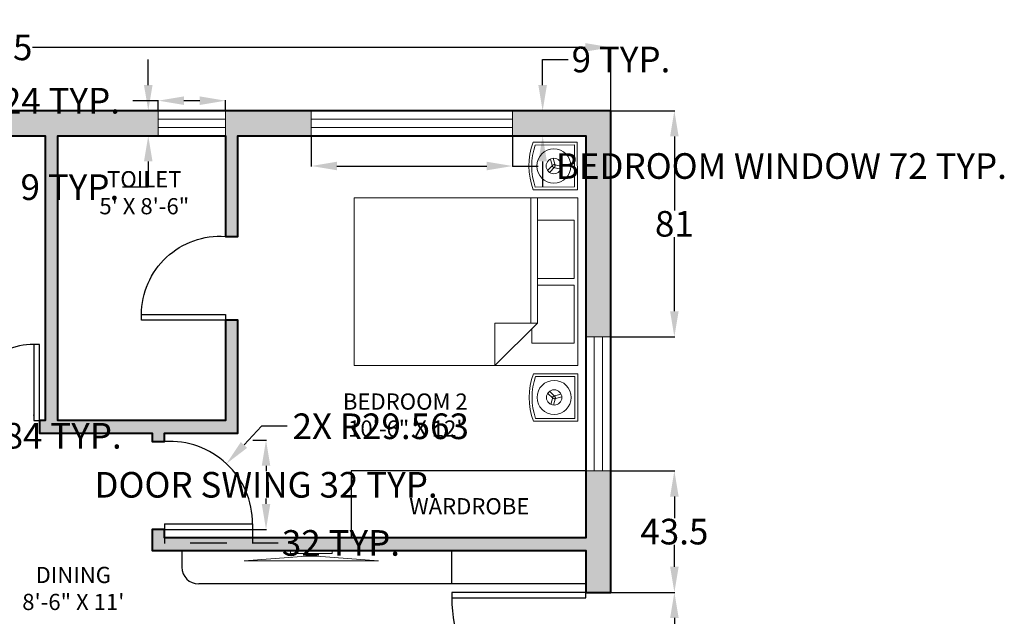
# Model space of a CAD drawing. Units: inches. Extents: x -51 to 563, y -59 to 453.
# Tile 6 of 6: x 211 to 563, y 240 to 453. Entities that reach past the tile are written whole.
import ezdxf

# ---------------------------------------------------------------- set-up
doc = ezdxf.new("R2010")
doc.units = ezdxf.units.IN
doc.header["$MEASUREMENT"] = 0
for name, color, linetype, lineweight in [('A-ANNO-DIMS', 2, 'Continuous', 18), ('A-ANNO-TEXT', 7, 'Continuous', 18), ('A-AREA-IDEN', 7, 'Continuous', 25), ('A-DOOR', 3, 'Continuous', 25), ('A-EQPM', 8, 'Continuous', 18), ('A-FLOR-CASE', 8, 'Continuous', 25), ('A-FURN', 8, 'Continuous', 18), ('A-GLAZ', 4, 'Continuous', 18), ('A-WALL', 7, 'Continuous', 40), ('A-WALL-PATT', 252, 'Continuous', 13)]:
    doc.layers.add(name, color=color, linetype=linetype, lineweight=lineweight)
doc.styles.get("Standard").update_dxf_attribs({"font": 'arial.ttf'})
doc.dimstyles.get("Standard").update_dxf_attribs({"dimtxt": 9.18, "dimasz": 9.18, "dimexe": 0.18, "dimexo": 0.0625, "dimgap": 0.09, "dimtad": 0, "dimtih": 1, "dimtoh": 1, "dimdec": 1, "dimzin": 0, "dimdsep": 46, "dimlunit": 3, "dimtxsty": 'Standard', "dimcen": 0.09, "dimadec": 0, "dimazin": 0, "dimtfac": 1, "dimtdec": 1, "dimtofl": 0, "dimtmove": 0, "dimatfit": 3, "dimfxl": 1, "dimtolj": 1, "dimtzin": 0, "dimarcsym": 0})

# ---------------------------------------------------------------- blocks, each defined once
blk = doc.blocks.new('Bed - Queen')
for p, q in [((0, -80.00003), (0, 0)), ((0, 0), (59.99999, 0)), ((59.99999, 0), (59.99999, -80.00003)), ((7.99999, -1.2), (28.79998, -1.2)), ((7.99999, -14.4), (7.99999, -1.2)), ((28.79998, -1.2), (28.79998, -14.4)), ((31.19999, -1.2), (51.99999, -1.2)), ((31.19999, -14.4), (31.19999, -1.2)), ((51.99999, -1.2), (51.99999, -16.4)), ((0, -14.4), (44.8, -14.4)), ((44.8, -16.8), (0, -16.8)), ((59.99999, -29.6), (44.8, -14.4)), ((44.8, -14.4), (44.8, -29.6)), ((51.99999, -16.4), (46.79936, -16.4)), ((44.8, -29.6), (59.99999, -29.6)), ((59.99999, -80.00003), (0, -80.00003))]:
    blk.add_line(p, q)
blk = doc.blocks.new('WIN-72IN')
for p, q in [((0, 0), (0, 9)), ((72, 0), (72, 9)), ((72, 6), (0, 6)), ((72, 3), (0, 3))]:
    blk.add_line(p, q)
blk = doc.blocks.new('WIN-48IN')
for p, q in [((9, 48), (0, 48)), ((3, 48), (3, 0)), ((6, 48), (6, 0)), ((9, 0), (0, 0))]:
    blk.add_line(p, q)
blk = doc.blocks.new('WIN-24IN')
for p, q in [((0, 0), (0, 9)), ((24, 0), (24, 9)), ((24, 6), (0, 6)), ((24, 3), (0, 3))]:
    blk.add_line(p, q)
blk = doc.blocks.new('DR-SWING-30IN')
for p, q in [((30, 30.07), (0, 30.07)), ((0, 30.07), (0, 28.07)), ((30, 28.07), (30, 30.07)), ((0, 28.07), (30, 28.07))]:
    blk.add_line(p, q)
blk.add_arc((28.07, 28.07), 28.07, 180, 273.9499)
blk = doc.blocks.new('DR-SWING-31_5IN')
for p, q in [((0, 2), (31.5, 2)), ((0, 2), (0, 0)), ((31.5, 2), (31.5, 0)), ((0, 0), (31.5, 0))]:
    blk.add_line(p, q)
blk.add_arc((1.94, 2), 29.56, 0, 93.7558)
blk = doc.blocks.new('TV-FLATSCREEN-48IN')
for p, q in [((0, 0), (22.17, 1.61)), ((48, 0), (25.84, 1.61)), ((0, 0), (48, 0))]:
    blk.add_line(p, q)
for points in [[(16.55, 3.67), (31.46, 3.67), (31.46, 2.61), (16.55, 2.61)], [(22.17, 2.61), (25.84, 2.61), (25.84, 1.61), (22.17, 1.61)]]:
    blk.add_lwpolyline(points, close=True)
blk = doc.blocks.new('*U11')
for p, q in [((-1.31, -0.61), (0.61, 1.31)), ((-0.61, -1.31), (1.31, 0.61))]:
    blk.add_line(p, q)
blk = doc.blocks.new('*U12')
at = {"color": 0, "linetype": 'ByBlock', "lineweight": -2, "transparency": 16777216}
for p, rotation in [((276.07, -10.08), 120), ((277.73, -11.74), 239.9999999999999)]:
    blk.add_blockref('*U11', p, dxfattribs=dict(at, rotation=rotation))
blk.add_blockref('*U11', (278.34, -9.47), dxfattribs=at)
blk = doc.blocks.new('TABLE-SIDE-WITH-LAMP')
for points in [[(17.03, 15.79), (17.03, 0), (0, 0), (0, 15.79, -0.18199)], [(16.03, 15.08), (16.03, 1), (1, 1), (1, 15.08, -0.16668)]]:
    blk.add_lwpolyline(points, format="xyb", close=True)
for centre, radius in [((8.51, 8.42), 6.11), ((8.51, 8.42), 2.75), ((8.51, 8.47), 0.5)]:
    blk.add_circle(centre, radius)
blk.add_blockref('*U12', (-268.87, 18.9))
blk = doc.blocks.new('WARDROBE-84X24IN')
for p, q in [((0, 24), (84, 24)), ((84, 24), (84, 0))]:
    blk.add_line(p, q)
blk = doc.blocks.new('*D39')
at = {"layer": 'A-ANNO-DIMS', "color": 0, "lineweight": -2, "transparency": 16777216}
for p, q in [((315.31, 411.79), (315.31, 400.87)), ((387.31, 411.79), (387.31, 400.87)), ((324.49, 401.05), (378.13, 401.05)), ((387.31, 401.05), (396.49, 401.05))]:
    blk.add_line(p, q, dxfattribs=at)
at = {"layer": 'A-ANNO-DIMS', "color": 0, "transparency": 16777216}
for points in [[(324.49, 402.58), (324.49, 399.52), (315.31, 401.05)], [(378.13, 402.58), (378.13, 399.52), (387.31, 401.05)]]:
    blk.add_solid(points, dxfattribs=at)
at = {"layer": 'Defpoints', "color": 0, "transparency": 16777216}
for p in [(315.31, 411.85), (387.31, 411.85), (387.31, 401.05)]:
    blk.add_point(p, dxfattribs=at)
at = {"layer": 'A-ANNO-DIMS', "color": 0, "transparency": 16777216, "insert": (483.55, 401.05), "char_height": 9.18, "attachment_point": 5}
blk.add_mtext('\\A1;BEDROOM WINDOW 72 TYP.', dxfattribs=at)
blk = doc.blocks.new('*D40')
at = {"layer": 'A-ANNO-DIMS', "color": 0, "lineweight": -2, "transparency": 16777216}
for p, q in [((398.11, 430.03), (398.11, 439.21)), ((398.11, 439.21), (407.29, 439.21)), ((387.37, 420.85), (398.29, 420.85)), ((387.37, 411.85), (398.29, 411.85)), ((398.11, 402.67), (398.11, 393.49))]:
    blk.add_line(p, q, dxfattribs=at)
at = {"layer": 'A-ANNO-DIMS', "color": 0, "transparency": 16777216}
for points in [[(396.58, 430.03), (399.64, 430.03), (398.11, 420.85)], [(396.58, 402.67), (399.64, 402.67), (398.11, 411.85)]]:
    blk.add_solid(points, dxfattribs=at)
at = {"layer": 'Defpoints', "color": 0, "transparency": 16777216}
for p in [(387.31, 420.85), (398.11, 420.85), (387.31, 411.85)]:
    blk.add_point(p, dxfattribs=at)
at = {"layer": 'A-ANNO-DIMS', "color": 0, "transparency": 16777216, "insert": (426.15, 439.21), "char_height": 9.18, "attachment_point": 5}
blk.add_mtext('\\A1;9 TYP.', dxfattribs=at)
blk = doc.blocks.new('*D41')
at = {"layer": 'A-ANNO-DIMS', "color": 0, "lineweight": -2, "transparency": 16777216}
for p, q in [((260.56, 424.45), (251.38, 424.45)), ((260.56, 420.91), (260.56, 424.63)), ((275.38, 424.45), (269.74, 424.45)), ((284.56, 420.91), (284.56, 424.63))]:
    blk.add_line(p, q, dxfattribs=at)
at = {"layer": 'A-ANNO-DIMS', "color": 0, "transparency": 16777216}
for points in [[(269.74, 425.98), (269.74, 422.92), (260.56, 424.45)], [(275.38, 425.98), (275.38, 422.92), (284.56, 424.45)]]:
    blk.add_solid(points, dxfattribs=at)
at = {"layer": 'Defpoints', "color": 0, "transparency": 16777216}
for p in [(260.56, 424.45), (260.56, 420.85), (284.56, 420.85)]:
    blk.add_point(p, dxfattribs=at)
at = {"layer": 'A-ANNO-DIMS', "color": 0, "transparency": 16777216, "insert": (180.35, 424.45), "char_height": 9.18, "attachment_point": 5}
blk.add_mtext('\\A1;BATH WINDOW 24 TYP.', dxfattribs=at)
blk = doc.blocks.new('*D42')
at = {"layer": 'A-ANNO-DIMS', "color": 0, "lineweight": -2, "transparency": 16777216}
for p, q in [((256.96, 430.03), (256.96, 439.21)), ((260.5, 420.85), (256.78, 420.85)), ((260.5, 411.85), (256.78, 411.85)), ((256.96, 402.67), (256.96, 393.49)), ((256.96, 393.49), (247.78, 393.49))]:
    blk.add_line(p, q, dxfattribs=at)
at = {"layer": 'A-ANNO-DIMS', "color": 0, "transparency": 16777216}
for points in [[(255.43, 430.03), (258.49, 430.03), (256.96, 420.85)], [(255.43, 402.67), (258.49, 402.67), (256.96, 411.85)]]:
    blk.add_solid(points, dxfattribs=at)
at = {"layer": 'Defpoints', "color": 0, "transparency": 16777216}
for p in [(260.56, 420.85), (256.96, 411.85), (260.56, 411.85)]:
    blk.add_point(p, dxfattribs=at)
at = {"layer": 'A-ANNO-DIMS', "color": 0, "transparency": 16777216, "insert": (228.91, 393.49), "char_height": 9.18, "attachment_point": 5}
blk.add_mtext('\\A1;9 TYP.', dxfattribs=at)
blk = doc.blocks.new('*D45')
at = {"layer": 'A-ANNO-DIMS', "color": 0, "lineweight": -2, "transparency": 16777216}
for p, q in [((294.37, 302.88), (299.29, 302.88)), ((299.11, 293.7), (299.11, 291.71)), ((299.11, 280.03), (299.11, 282.02)), ((294.37, 270.85), (299.29, 270.85))]:
    blk.add_line(p, q, dxfattribs=at)
at = {"layer": 'A-ANNO-DIMS', "color": 0, "transparency": 16777216}
for points in [[(297.58, 293.7), (300.64, 293.7), (299.11, 302.88)], [(297.58, 280.03), (300.64, 280.03), (299.11, 270.85)]]:
    blk.add_solid(points, dxfattribs=at)
at = {"layer": 'Defpoints', "color": 0, "transparency": 16777216}
for p in [(294.31, 302.88), (299.11, 302.88), (294.31, 270.85)]:
    blk.add_point(p, dxfattribs=at)
at = {"layer": 'A-ANNO-DIMS', "color": 0, "transparency": 16777216, "insert": (299.11, 286.87), "char_height": 9.18, "attachment_point": 5}
blk.add_mtext('\\A1;DOOR SWING 32 TYP.', dxfattribs=at)
blk = doc.blocks.new('*D46')
at = {"layer": 'A-ANNO-DIMS', "color": 0, "lineweight": -2, "transparency": 16777216}
for p, q in [((262.81, 270.79), (262.81, 265.86)), ((294.31, 270.79), (294.31, 265.86)), ((271.99, 266.04), (285.13, 266.04)), ((294.31, 266.04), (303.49, 266.04))]:
    blk.add_line(p, q, dxfattribs=at)
at = {"layer": 'A-ANNO-DIMS', "color": 0, "transparency": 16777216}
for points in [[(271.99, 267.57), (271.99, 264.51), (262.81, 266.04)], [(285.13, 267.57), (285.13, 264.51), (294.31, 266.04)]]:
    blk.add_solid(points, dxfattribs=at)
at = {"layer": 'Defpoints', "color": 0, "transparency": 16777216}
for p in [(262.81, 270.85), (294.31, 270.85), (294.31, 266.04)]:
    blk.add_point(p, dxfattribs=at)
at = {"layer": 'A-ANNO-DIMS', "color": 0, "transparency": 16777216, "insert": (325.92, 266.04), "char_height": 9.18, "attachment_point": 5}
blk.add_mtext('\\A1;32 TYP.', dxfattribs=at)
blk = doc.blocks.new('*D47')
at = {"layer": 'A-ANNO-DIMS', "color": 0, "lineweight": -2, "transparency": 16777216}
for p, q in [((35.56, 291.91), (35.56, 304.63)), ((44.74, 304.45), (110.38, 304.45)), ((119.56, 291.91), (119.56, 304.63)), ((119.56, 304.45), (128.74, 304.45))]:
    blk.add_line(p, q, dxfattribs=at)
at = {"layer": 'A-ANNO-DIMS', "color": 0, "transparency": 16777216}
for points in [[(44.74, 305.98), (44.74, 302.92), (35.56, 304.45)], [(110.38, 305.98), (110.38, 302.92), (119.56, 304.45)]]:
    blk.add_solid(points, dxfattribs=at)
at = {"layer": 'Defpoints', "color": 0, "transparency": 16777216}
for p in [(119.56, 304.45), (35.56, 291.85), (119.56, 291.85)]:
    blk.add_point(p, dxfattribs=at)
at = {"layer": 'A-ANNO-DIMS', "color": 0, "transparency": 16777216, "insert": (190.9, 304.45), "char_height": 9.18, "attachment_point": 5}
blk.add_mtext('\\A1;WARDROBE 84 TYP.', dxfattribs=at)
blk = doc.blocks.new('*D65')
at = {"layer": 'A-ANNO-DIMS', "color": 0, "lineweight": -2, "transparency": 16777216}
for p, q in [((-12.44, 272.41), (-12.44, 443.73)), ((-3.26, 443.55), (194.61, 443.55)), ((413.38, 443.55), (215.51, 443.55)), ((422.56, 420.91), (422.56, 443.73))]:
    blk.add_line(p, q, dxfattribs=at)
at = {"layer": 'A-ANNO-DIMS', "color": 0, "transparency": 16777216}
for points in [[(-3.26, 445.08), (-3.26, 442.02), (-12.44, 443.55)], [(413.38, 445.08), (413.38, 442.02), (422.56, 443.55)]]:
    blk.add_solid(points, dxfattribs=at)
at = {"layer": 'Defpoints', "color": 0, "transparency": 16777216}
for p in [(422.56, 443.55), (422.56, 420.85), (-12.44, 272.35)]:
    blk.add_point(p, dxfattribs=at)
at = {"layer": 'A-ANNO-DIMS', "color": 0, "transparency": 16777216, "insert": (205.06, 443.55), "char_height": 9.18, "attachment_point": 5}
blk.add_mtext('\\A1;435', dxfattribs=at)
blk = doc.blocks.new('*D68')
at = {"layer": 'A-ANNO-DIMS', "color": 0, "lineweight": -2, "transparency": 16777216}
for p, q in [((422.62, 420.85), (445.44, 420.85)), ((445.26, 411.67), (445.26, 385.12)), ((445.26, 349.03), (445.26, 375.57)), ((422.62, 339.85), (445.44, 339.85))]:
    blk.add_line(p, q, dxfattribs=at)
at = {"layer": 'A-ANNO-DIMS', "color": 0, "transparency": 16777216}
for points in [[(443.73, 411.67), (446.79, 411.67), (445.26, 420.85)], [(443.73, 349.03), (446.79, 349.03), (445.26, 339.85)]]:
    blk.add_solid(points, dxfattribs=at)
at = {"layer": 'Defpoints', "color": 0, "transparency": 16777216}
for p in [(422.56, 420.85), (422.56, 339.85), (445.26, 339.85)]:
    blk.add_point(p, dxfattribs=at)
at = {"layer": 'A-ANNO-DIMS', "color": 0, "transparency": 16777216, "insert": (445.26, 380.35), "char_height": 9.18, "attachment_point": 5}
blk.add_mtext('\\A1;81', dxfattribs=at)
blk = doc.blocks.new('*D69')
at = {"layer": 'A-ANNO-DIMS', "color": 0, "lineweight": -2, "transparency": 16777216}
for p, q in [((422.62, 291.85), (445.44, 291.85)), ((445.26, 282.67), (445.26, 274.88)), ((445.26, 257.53), (445.26, 265.32)), ((422.62, 248.35), (445.44, 248.35))]:
    blk.add_line(p, q, dxfattribs=at)
at = {"layer": 'A-ANNO-DIMS', "color": 0, "transparency": 16777216}
for points in [[(443.73, 282.67), (446.79, 282.67), (445.26, 291.85)], [(443.73, 257.53), (446.79, 257.53), (445.26, 248.35)]]:
    blk.add_solid(points, dxfattribs=at)
at = {"layer": 'Defpoints', "color": 0, "transparency": 16777216}
for p in [(422.56, 291.85), (422.56, 248.35), (445.26, 248.35)]:
    blk.add_point(p, dxfattribs=at)
at = {"layer": 'A-ANNO-DIMS', "color": 0, "transparency": 16777216, "insert": (445.26, 270.1), "char_height": 9.18, "attachment_point": 5}
blk.add_mtext('\\A1;43.5', dxfattribs=at)
blk = doc.blocks.new('*D70')
at = {"layer": 'A-ANNO-DIMS', "color": 0, "lineweight": -2, "transparency": 16777216}
for p, q in [((422.62, 248.35), (445.44, 248.35)), ((445.26, 239.17), (445.26, 229.12)), ((445.26, 209.53), (445.26, 219.57)), ((422.62, 200.35), (445.44, 200.35))]:
    blk.add_line(p, q, dxfattribs=at)
at = {"layer": 'A-ANNO-DIMS', "color": 0, "transparency": 16777216}
for points in [[(443.73, 239.17), (446.79, 239.17), (445.26, 248.35)], [(443.73, 209.53), (446.79, 209.53), (445.26, 200.35)]]:
    blk.add_solid(points, dxfattribs=at)
at = {"layer": 'Defpoints', "color": 0, "transparency": 16777216}
for p in [(422.56, 248.35), (422.56, 200.35), (445.26, 200.35)]:
    blk.add_point(p, dxfattribs=at)
at = {"layer": 'A-ANNO-DIMS', "color": 0, "transparency": 16777216, "insert": (445.26, 224.35), "char_height": 9.18, "attachment_point": 5}
blk.add_mtext('\\A1;48', dxfattribs=at)
blk = doc.blocks.new('*D81')
at = {"layer": 'A-ANNO-DIMS', "color": 0, "lineweight": -2, "transparency": 16777216}
for p, q in [((411.51, 246.35), (411.69, 246.35)), ((411.6, 246.26), (411.6, 246.44)), ((360.63, 193.16), (373.39, 206.48)), ((351.45, 193.16), (360.63, 193.16))]:
    blk.add_line(p, q, dxfattribs=at)
at = {"layer": 'A-ANNO-DIMS', "color": 0, "transparency": 16777216}
blk.add_solid([(372.29, 207.54), (374.5, 205.42), (379.74, 213.11)], dxfattribs=at)
at = {"layer": 'Defpoints', "color": 0, "transparency": 16777216}
for p in [(411.6, 246.35), (379.74, 213.11)]:
    blk.add_point(p, dxfattribs=at)
at = {"layer": 'A-ANNO-DIMS', "color": 0, "transparency": 16777216, "insert": (331.5, 193.16), "char_height": 9.18, "attachment_point": 5}
blk.add_mtext('\\A1;R46.04', dxfattribs=at)
blk = doc.blocks.new('*D83')
at = {"layer": 'A-ANNO-DIMS', "color": 0, "lineweight": -2, "transparency": 16777216}
for p, q in [((174.81, 341.48), (183.99, 341.48)), ((183.99, 341.48), (190.73, 335.25)), ((215.97, 311.82), (216.15, 311.82)), ((216.06, 311.73), (216.06, 311.91))]:
    blk.add_line(p, q, dxfattribs=at)
at = {"layer": 'A-ANNO-DIMS', "color": 0, "transparency": 16777216}
blk.add_solid([(191.76, 336.37), (189.69, 334.13), (197.46, 329.02)], dxfattribs=at)
at = {"layer": 'Defpoints', "color": 0, "transparency": 16777216}
for p in [(197.46, 329.02), (216.06, 311.82)]:
    blk.add_point(p, dxfattribs=at)
at = {"layer": 'A-ANNO-DIMS', "color": 0, "transparency": 16777216, "insert": (151.27, 341.48), "char_height": 9.18, "attachment_point": 5}
blk.add_mtext('\\A1;R25.327', dxfattribs=at)
blk = doc.blocks.new('*D84')
at = {"layer": 'A-ANNO-DIMS', "color": 0, "lineweight": -2, "transparency": 16777216}
for p, q in [((297.5, 307.83), (291.23, 301.13)), ((306.68, 307.83), (297.5, 307.83)), ((264.65, 272.85), (264.83, 272.85)), ((264.74, 272.76), (264.74, 272.94))]:
    blk.add_line(p, q, dxfattribs=at)
at = {"layer": 'A-ANNO-DIMS', "color": 0, "transparency": 16777216}
blk.add_solid([(290.11, 302.17), (292.34, 300.08), (284.95, 294.43)], dxfattribs=at)
at = {"layer": 'Defpoints', "color": 0, "transparency": 16777216}
for p in [(284.95, 294.43), (264.74, 272.85)]:
    blk.add_point(p, dxfattribs=at)
at = {"layer": 'A-ANNO-DIMS', "color": 0, "transparency": 16777216, "insert": (340.16, 307.83), "char_height": 9.18, "attachment_point": 5}
blk.add_mtext('\\A1;2X R29.563', dxfattribs=at)

msp = doc.modelspace()

# ---------------------------------------------------------------- linework, layer by layer
at = {"layer": 'A-DOOR'}
for p, q in [((218.0584, 337.1479), (216.0584, 337.1479)), ((216.0584, 337.1479), (216.0584, 309.8479)), ((218.0584, 309.8479), (218.0584, 337.1479)), ((216.0584, 309.8479), (218.0584, 309.8479)), ((413.5584, 248.3479), (365.5584, 248.3479)), ((365.5584, 248.3479), (365.5584, 246.3479)), ((413.5584, 246.3479), (413.5584, 248.3479)), ((365.5584, 246.3479), (413.5584, 246.3479))]:
    msp.add_line(p, q, dxfattribs=at)
for centre, radius, start, end in [((216.0584, 311.8209), 25.327, 90, 184.468005), ((411.6, 246.3479), 46.0417, 180, 272.43775)]:
    msp.add_arc(centre, radius, start, end, dxfattribs=at)
at = {"layer": 'A-FLOR-CASE'}
for p, q in [((269.0074, 263.3479), (269.0074, 257.3479)), ((365.5584, 251.3479), (365.5584, 263.3479)), ((413.5584, 251.3479), (275.0074, 251.3479))]:
    msp.add_line(p, q, dxfattribs=at)
msp.add_arc((275.0074, 257.3479), 6, 180, 270, dxfattribs=at)
at = {"layer": 'A-WALL'}
msp.add_lwpolyline([(160.0584, 411.8479), (220.0584, 411.8479), (220.0584, 309.8479), (218.0584, 309.8479), (218.0584, 305.3479), (220.0584, 305.3479), (258.3084, 305.3479), (258.3084, 302.3479), (262.8084, 302.3479), (262.8084, 305.3479), (284.5584, 305.3479), (289.0584, 305.3479), (289.0584, 345.8479), (284.5584, 345.8479), (284.5584, 309.8479), (224.5584, 309.8479), (224.5584, 411.8479), (284.5584, 411.8479), (284.5584, 375.8479), (289.0584, 375.8479), (289.0584, 411.8479), (413.5584, 411.8479), (413.5584, 267.8479), (262.8084, 267.8479), (262.8084, 270.8479), (258.3084, 270.8479), (258.3084, 267.8479), (258.3084, 263.3479), (413.5584, 263.3479), (413.5584, 248.3479), (422.5584, 248.3479), (422.5584, 420.8479), (26.5584, 420.8479)], dxfattribs=at)
at = {"layer": 'A-WALL-PATT'}
for points in [[(184.0584, 420.8479), (184.0584, 411.8479), (260.5584, 420.8479), (260.5584, 411.8479)], [(315.3084, 420.8479), (315.3084, 411.8479), (284.5584, 420.8479), (289.0584, 411.8479)], [(284.5584, 420.8479), (289.0584, 411.8479), (284.5584, 375.8479), (289.0584, 375.8479)], [(413.5584, 411.8479), (422.5584, 420.8479), (387.3084, 411.8479), (387.3084, 420.8479)], [(413.5584, 339.8479), (422.5584, 339.8479), (413.5584, 411.8479), (422.5584, 420.8479)], [(220.0584, 309.8479), (224.5584, 309.8479), (220.0584, 411.8479), (224.5584, 411.8479)], [(284.5584, 345.8479), (289.0584, 345.8479), (284.5584, 309.8479), (289.0584, 305.3479)], [(284.5584, 309.8479), (289.0584, 305.3479), (218.0584, 309.8479), (218.0584, 305.3479)], [(258.3084, 305.3479), (258.3084, 302.3479), (262.8084, 305.3479), (262.8084, 302.3479)], [(413.5584, 248.3479), (422.5584, 248.3479), (413.5584, 291.8479), (422.5584, 291.8479)], [(258.3084, 263.3479), (262.8084, 267.8479), (258.3084, 270.8479), (262.8084, 270.8479)], [(413.5584, 263.3479), (413.5584, 267.8479), (258.3084, 263.3479), (262.8084, 267.8479)]]:
    msp.add_solid(points, dxfattribs=at)

# ---------------------------------------------------------------- block references
at = {"layer": 'A-DOOR', "extrusion": (0, 0, -1), "zscale": -1, "rotation": 180}
msp.add_blockref('DR-SWING-30IN', (-254.558, 375.9138), dxfattribs=at)
at = {"layer": 'A-DOOR'}
msp.add_blockref('DR-SWING-31_5IN', (262.808, 270.848), dxfattribs=at)
at = {"layer": 'A-EQPM'}
msp.add_blockref('TV-FLATSCREEN-48IN', (291.3258, 259.675), dxfattribs=at)
at = {"layer": 'A-FLOR-CASE', "extrusion": (0, 0, -1), "zscale": -1}
msp.add_blockref('WARDROBE-84X24IN', (-413.5587, 267.848), dxfattribs=at)
at = {"layer": 'A-FURN', "extrusion": (0, 0, -1), "zscale": -1, "rotation": 269.8554367965242}
msp.add_blockref('TABLE-SIDE-WITH-LAMP', (-410.5241, 409.5879), dxfattribs=at)
at = {"layer": 'A-FURN'}
for name, p, rotation in [('Bed - Queen', (410.6498, 389.6145), 270), ('TABLE-SIDE-WITH-LAMP', (410.6502, 309.6409), 89.99999999999996)]:
    msp.add_blockref(name, p, dxfattribs=dict(at, rotation=rotation))
at = {"layer": 'A-GLAZ', "rotation": 180}
for name, p in [('WIN-24IN', (284.5587, 420.8478)), ('WIN-48IN', (422.5587, 339.8478))]:
    msp.add_blockref(name, p, dxfattribs=at)
at = {"layer": 'A-GLAZ'}
msp.add_blockref('WIN-72IN', (315.308, 411.848), dxfattribs=at)

# ---------------------------------------------------------------- texts
at = {"layer": 'A-ANNO-TEXT', "insert": (347.0672, 282.0858), "char_height": 5.8, "attachment_point": 1}
msp.add_mtext_dynamic_manual_height_columns('\\pxqc;WARDROBE', width=49.588896, gutter_width=1, heights=[0], dxfattribs=at)
at = {"layer": 'A-AREA-IDEN', "char_height": 5.8, "attachment_point": 1}
for s, width, insert in [('\\pxqc;TOILET\\P5\' X 8\'-6"', 33.368061, (238.8604, 399.2245)), ('\\pxqc;BEDROOM 2\\P10\'-6" X 12\'', 49.588896, (324.169, 319.59)), ('\\pxqc;DINING\\P8\'-6" X 11\'', 49.588896, (205.3304, 257.481))]:
    msp.add_mtext_dynamic_manual_height_columns(s, width=width, gutter_width=1, heights=[0], dxfattribs=dict(at, insert=insert))

# ---------------------------------------------------------------- dimensions: what is measured, and where the dimension line sits
at = {"layer": 'A-ANNO-DIMS'}
for base, p1, p2, angle, text, picture, middle in [((260.5584, 424.4479), (284.5584, 420.8479), (260.5584, 420.8479), 180, 'BATH WINDOW <> TYP.', '*D41', (180.35, 424.4479)), ((398.1084, 420.8479), (387.3084, 411.8479), (387.3084, 420.8479), 90, '<> TYP.', '*D40', (426.1548, 439.2079)), ((256.9584, 411.8479), (260.5584, 420.8479), (260.5584, 411.8479), 270, '<> TYP.', '*D42', (228.9119, 393.4879)), ((299.1137, 302.8835), (294.3084, 270.8479), (294.3084, 302.8835), 90, 'DOOR SWING <> TYP.', '*D45', (299.1137, 286.8657))]:
    dim = msp.add_linear_dim(base=base, p1=p1, p2=p2, angle=angle, text=text, dimstyle='Standard', override={"dimdec": 0, "dimlfac": 1, "dimrnd": 0, "dimzin": 0, "dimdsep": 46, "dimlunit": 2}, dxfattribs=at)
    dim.commit()
    dim.dimension.update_dxf_attribs({"geometry": picture, "text_midpoint": middle})
dim = msp.add_linear_dim(base=(422.5584, 443.5479), p1=(-12.4416, 272.3479), p2=(422.5584, 420.8479), dimstyle='Standard', override={"dimdec": 0, "dimlfac": 1, "dimrnd": 0, "dimzin": 0, "dimdsep": 46, "dimlunit": 2}, dxfattribs=at)
dim.commit()
dim.dimension.update_dxf_attribs({"geometry": '*D65', "text_midpoint": (205.0584, 443.5479)})
for base, p1, p2, text, picture, middle in [((387.3084, 401.0479), (315.3084, 411.8479), (387.3084, 411.8479), 'BEDROOM WINDOW <> TYP.', '*D39', (483.5473, 401.0479)), ((119.5584, 304.4479), (35.5584, 291.8479), (119.5584, 291.8479), 'WARDROBE <> TYP.', '*D47', (190.903, 304.4479)), ((294.3083684352, 266.0425555457), (262.8083684352, 270.8478991093), (294.3083684352, 270.8478991093), '<> TYP.', '*D46', (325.9178295539, 266.0425555457))]:
    dim = msp.add_linear_dim(base=base, p1=p1, p2=p2, text=text, dimstyle='Standard', override={"dimdec": 0, "dimlfac": 1, "dimrnd": 0, "dimzin": 0, "dimdsep": 46, "dimlunit": 2}, dxfattribs=at)
    dim.commit()
    dim.dimension.update_dxf_attribs({"geometry": picture, "text_midpoint": middle})
for base, p1, p2, override, picture, middle in [((445.2584, 339.8479), (422.5584, 420.8479), (422.5584, 339.8479), {"dimdec": 0, "dimlfac": 1, "dimrnd": 0, "dimzin": 0, "dimdsep": 46, "dimlunit": 2}, '*D68', (445.2584, 380.3479)), ((445.2584, 248.3479), (422.5584, 291.8479), (422.5584, 248.3479), {"dimdec": 1, "dimlfac": 1, "dimrnd": 0, "dimzin": 0, "dimdsep": 46, "dimlunit": 2}, '*D69', (445.2584, 270.0979)), ((445.2584, 200.3479), (422.5584, 248.3479), (422.5584, 200.3479), {"dimdec": 0, "dimlfac": 1, "dimrnd": 0, "dimzin": 0, "dimdsep": 46, "dimlunit": 2}, '*D70', (445.2584, 224.3479))]:
    dim = msp.add_linear_dim(base=base, p1=p1, p2=p2, angle=90, dimstyle='Standard', override=override, dxfattribs=at)
    dim.commit()
    dim.dimension.update_dxf_attribs({"geometry": picture, "text_midpoint": middle})
dim = msp.add_radius_dim(center=(216.0584, 311.8209), mpoint=(197.465, 329.018), dimstyle='Standard', override={"dimdec": 3, "dimlfac": 1, "dimrnd": 0, "dimzin": 0, "dimdsep": 46, "dimlunit": 2}, dxfattribs=at)
dim.commit()
dim.dimension.update_dxf_attribs({"geometry": '*D83', "text_midpoint": (151.2684, 341.4845)})
dim = msp.add_radius_dim(center=(264.7449, 272.8479), mpoint=(284.9532, 294.4262), text='2X <>', dimstyle='Standard', override={"dimdec": 3, "dimlfac": 1, "dimrnd": 0, "dimzin": 0, "dimdsep": 46, "dimlunit": 2}, dxfattribs=at)
dim.commit()
dim.dimension.update_dxf_attribs({"geometry": '*D84', "text_midpoint": (340.162, 307.8271)})
dim = msp.add_radius_dim(center=(411.6, 246.3479), mpoint=(379.744, 213.106), dimstyle='Standard', override={"dimdec": 2, "dimlfac": 1, "dimrnd": 0, "dimzin": 0, "dimdsep": 46, "dimlunit": 2}, dxfattribs=at)
dim.commit()
dim.dimension.update_dxf_attribs({"geometry": '*D81', "text_midpoint": (331.4975, 193.1608), "dimtype": 164})

doc.saveas('drawing.dxf')
